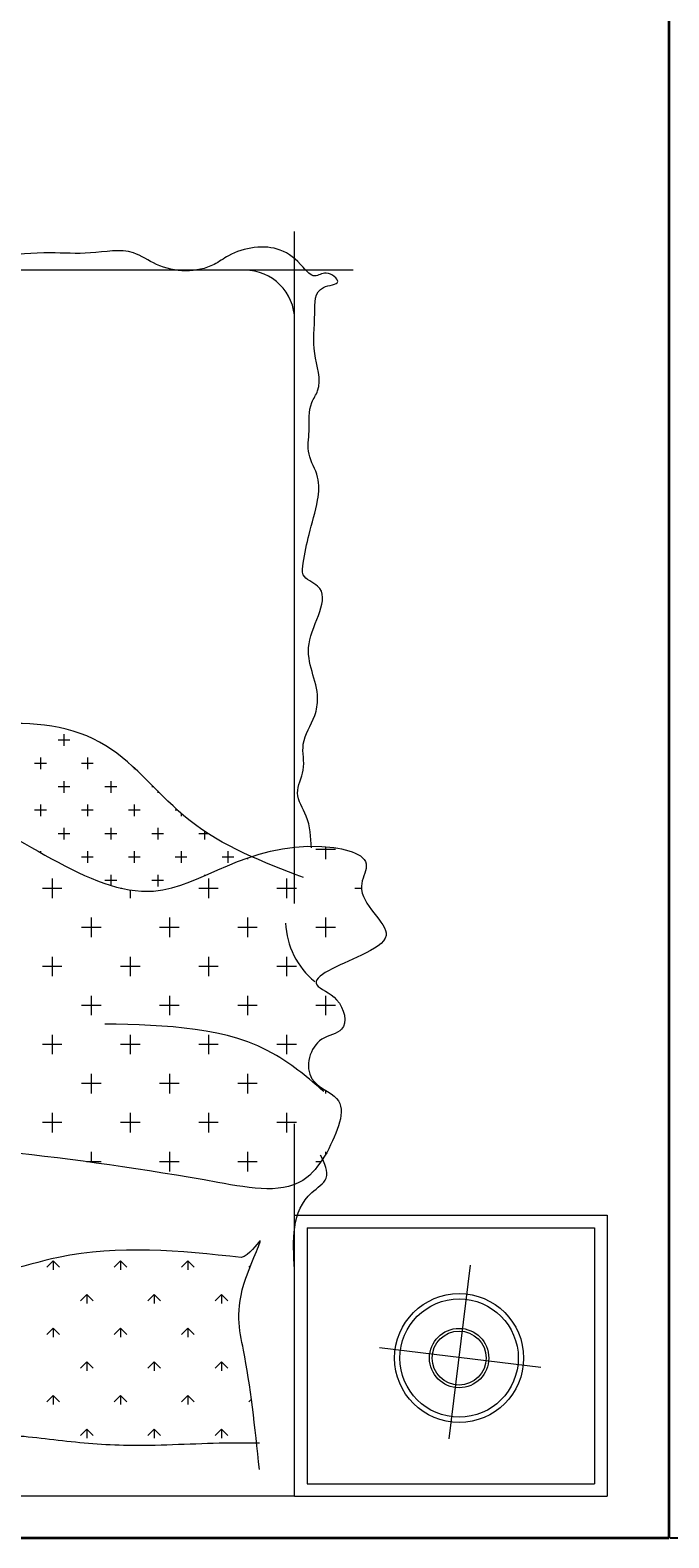
# Model space of a CAD drawing. Units: inches. Extents: x 3731 to 4318, y 1310 to 2388.
# Tile 46 of 57: x 4192 to 4234, y 1943 to 2043. Entities that reach past the tile are written whole.
import ezdxf

# ---------------------------------------------------------------- set-up
doc = ezdxf.new("R2010")
doc.units = ezdxf.units.IN
for name, color, linetype, lineweight in [('A-ANNO-DIMS', 2, 'Continuous', 18), ('A-FURN', 8, 'Continuous', 13), ('A-WALL', 7, 'Continuous', 35)]:
    doc.layers.add(name, color=color, linetype=linetype, lineweight=lineweight)
doc.styles.get("Standard").update_dxf_attribs({"font": 'arial.ttf'})
doc.dimstyles.get("Standard").update_dxf_attribs({"dimtxt": 0.18, "dimasz": 0.18, "dimexe": 0.18, "dimexo": 0.0625, "dimgap": 0.09, "dimtad": 0, "dimtih": 1, "dimtoh": 1, "dimdec": 4, "dimzin": 0, "dimdsep": 46, "dimtxsty": 'Standard', "dimcen": 0.09, "dimadec": 0, "dimazin": 0, "dimtfac": 1, "dimtdec": 4, "dimtofl": 0, "dimtmove": 0, "dimatfit": 3, "dimfxl": 1, "dimtolj": 1, "dimtzin": 0, "dimarcsym": 0})

# ---------------------------------------------------------------- blocks, each defined once
blk = doc.blocks.new('A$C200C7901')
for p, q in [((0, 1.8834), (0, 2.3334)), ((0.5, 2.3334), (0, 2.3334)), ((0.5, 2.3334), (0.5, 1.7369)), ((0.5, 2.3334), (0.5, 1.7369)), ((0.5, 2.3334), (2, 2.3334)), ((0.5701, 1.9635), (0.5733, 1.9666)), ((0.5701, 1.9635), (0.5733, 1.9666)), ((0.5, 1.8834), (0, 1.8834)), ((0.4504, 1.782), (0.4504, 1.7863)), ((0.4504, 1.782), (0.4504, 1.7863)), ((0.458, 1.7977), (0.466, 1.7977)), ((0.458, 1.7977), (0.466, 1.7977)), ((0.4504, 1.6834), (0.4504, 1.6883)), ((0.4504, 1.6834), (0.4504, 1.6883)), ((0.4656, 1.6727), (0.466, 1.6727)), ((0.4656, 1.6727), (0.466, 1.6727)), ((0.5597, 1.6727), (0.591, 1.6727)), ((0.5597, 1.6727), (0.591, 1.6727)), ((0.4347, 1.5477), (0.466, 1.5477)), ((0.4504, 1.532), (0.4504, 1.5633)), ((0.6847, 1.5477), (0.716, 1.5477)), ((0.4347, 1.4227), (0.466, 1.4227)), ((0.5, 1.3845), (0.5, 0.3086)), ((0.3931, 1.3602), (0.4035, 1.3602)), ((0.3931, 1.3602), (0.4035, 1.3602)), ((0.4972, 1.3602), (0.5285, 1.3602)), ((0.4972, 1.3602), (0.5285, 1.3602)), ((0.4504, 1.2936), (0.4504, 1.3133)), ((0.4504, 1.2936), (0.4504, 1.3133)), ((0.4347, 1.2977), (0.466, 1.2977)), ((0.4347, 1.2977), (0.466, 1.2977)), ((0.4061, 0.3703), (2.0386, 0.3703))]:
    blk.add_line(p, q)
at = {"linetype": 'ByBlock'}
for p, q in [((0.02, 1.9034), (0.02, 2.3134)), ((0.48, 2.3134), (0.02, 2.3134)), ((0.48, 1.9034), (0.48, 2.3134)), ((0.2524, 2.2412), (0.2186, 1.9635)), ((0.6171, 2.2259), (0.607, 2.236)), ((0.6171, 2.2259), (0.607, 2.236)), ((0.6171, 2.2259), (0.6171, 2.2402)), ((0.6171, 2.2259), (0.6171, 2.2402)), ((0.6171, 2.2259), (0.6272, 2.236)), ((0.6171, 2.2259), (0.6272, 2.236)), ((0.7249, 2.2259), (0.7148, 2.236)), ((0.7249, 2.2259), (0.7148, 2.236)), ((0.7249, 2.2259), (0.7249, 2.2402)), ((0.7249, 2.2259), (0.7249, 2.2402)), ((0.7249, 2.2259), (0.735, 2.236)), ((0.7249, 2.2259), (0.735, 2.236)), ((0.8326, 2.2259), (0.8225, 2.236)), ((0.8326, 2.2259), (0.8225, 2.236)), ((0.8326, 2.2259), (0.8326, 2.2402)), ((0.8326, 2.2259), (0.8326, 2.2402)), ((0.8326, 2.2259), (0.8427, 2.236)), ((0.8326, 2.2259), (0.8427, 2.236)), ((0.5692, 2.178), (0.5733, 2.1822)), ((0.5692, 2.178), (0.5733, 2.1822)), ((0.671, 2.1721), (0.6609, 2.1822)), ((0.671, 2.1721), (0.6609, 2.1822)), ((0.671, 2.172), (0.671, 2.1863)), ((0.671, 2.172), (0.671, 2.1863)), ((0.671, 2.1721), (0.6811, 2.1822)), ((0.671, 2.1721), (0.6811, 2.1822)), ((0.7787, 2.1721), (0.7686, 2.1822)), ((0.7787, 2.1721), (0.7686, 2.1822)), ((0.7787, 2.172), (0.7787, 2.1863)), ((0.7787, 2.172), (0.7787, 2.1863)), ((0.7787, 2.1721), (0.7889, 2.1822)), ((0.7787, 2.1721), (0.7889, 2.1822)), ((0.8865, 2.1721), (0.8764, 2.1822)), ((0.8865, 2.1721), (0.8764, 2.1822)), ((0.8865, 2.172), (0.8865, 2.1863)), ((0.8865, 2.172), (0.8865, 2.1863)), ((0.8865, 2.1721), (0.8966, 2.1822)), ((0.8865, 2.1721), (0.8966, 2.1822)), ((0.3641, 2.0951), (0.1061, 2.1268)), ((0.6171, 2.1182), (0.607, 2.1283)), ((0.6171, 2.1182), (0.607, 2.1283)), ((0.6171, 2.1182), (0.6171, 2.1325)), ((0.6171, 2.1182), (0.6171, 2.1325)), ((0.6171, 2.1182), (0.6272, 2.1283)), ((0.6171, 2.1182), (0.6272, 2.1283)), ((0.7249, 2.1182), (0.7148, 2.1283)), ((0.7249, 2.1182), (0.7148, 2.1283)), ((0.7249, 2.1182), (0.7249, 2.1325)), ((0.7249, 2.1182), (0.7249, 2.1325)), ((0.7249, 2.1182), (0.735, 2.1283)), ((0.7249, 2.1182), (0.735, 2.1283)), ((0.8326, 2.1182), (0.8225, 2.1283)), ((0.8326, 2.1182), (0.8225, 2.1283)), ((0.8326, 2.1182), (0.8326, 2.1325)), ((0.8326, 2.1182), (0.8326, 2.1325)), ((0.8326, 2.1182), (0.8427, 2.1283)), ((0.8326, 2.1182), (0.8427, 2.1283)), ((0.671, 2.0643), (0.671, 2.0786)), ((0.671, 2.0643), (0.671, 2.0786)), ((0.7787, 2.0643), (0.7787, 2.0786)), ((0.7787, 2.0643), (0.7787, 2.0786)), ((0.8865, 2.0643), (0.8865, 2.0786)), ((0.8865, 2.0643), (0.8865, 2.0786)), ((0.671, 2.0643), (0.6609, 2.0744)), ((0.671, 2.0643), (0.6609, 2.0744)), ((0.671, 2.0643), (0.6811, 2.0744)), ((0.671, 2.0643), (0.6811, 2.0744)), ((0.7787, 2.0643), (0.7686, 2.0744)), ((0.7787, 2.0643), (0.7686, 2.0744)), ((0.7787, 2.0643), (0.7889, 2.0744)), ((0.7787, 2.0643), (0.7889, 2.0744)), ((0.8865, 2.0643), (0.8764, 2.0744)), ((0.8865, 2.0643), (0.8764, 2.0744)), ((0.8865, 2.0643), (0.8966, 2.0744)), ((0.8865, 2.0643), (0.8966, 2.0744)), ((0.6171, 2.0104), (0.607, 2.0205)), ((0.6171, 2.0104), (0.607, 2.0205)), ((0.6171, 2.0104), (0.6171, 2.0247)), ((0.6171, 2.0104), (0.6171, 2.0247)), ((0.6171, 2.0104), (0.6272, 2.0205)), ((0.6171, 2.0104), (0.6272, 2.0205)), ((0.7249, 2.0104), (0.7148, 2.0205)), ((0.7249, 2.0104), (0.7148, 2.0205)), ((0.7249, 2.0104), (0.7249, 2.0247)), ((0.7249, 2.0104), (0.7249, 2.0247)), ((0.7249, 2.0104), (0.735, 2.0205)), ((0.7249, 2.0104), (0.735, 2.0205)), ((0.8326, 2.0104), (0.8225, 2.0205)), ((0.8326, 2.0104), (0.8225, 2.0205)), ((0.8326, 2.0104), (0.8326, 2.0247)), ((0.8326, 2.0104), (0.8326, 2.0247)), ((0.8326, 2.0104), (0.8427, 2.0205)), ((0.8326, 2.0104), (0.8427, 2.0205)), ((0.671, 1.9565), (0.6609, 1.9666)), ((0.671, 1.9565), (0.6609, 1.9666)), ((0.671, 1.9565), (0.671, 1.9708)), ((0.671, 1.9565), (0.671, 1.9708)), ((0.671, 1.9565), (0.6811, 1.9666)), ((0.671, 1.9565), (0.6811, 1.9666)), ((0.7787, 1.9565), (0.7686, 1.9666)), ((0.7787, 1.9565), (0.7686, 1.9666)), ((0.7787, 1.9565), (0.7787, 1.9708)), ((0.7787, 1.9565), (0.7787, 1.9708)), ((0.7787, 1.9565), (0.7889, 1.9666)), ((0.7787, 1.9565), (0.7889, 1.9666)), ((0.8865, 1.9565), (0.8764, 1.9666)), ((0.8865, 1.9565), (0.8764, 1.9666)), ((0.8865, 1.9565), (0.8865, 1.9708)), ((0.8865, 1.9565), (0.8865, 1.9708)), ((0.8865, 1.9565), (0.8966, 1.9666)), ((0.8865, 1.9565), (0.8966, 1.9666)), ((0.48, 1.9034), (0.02, 1.9034)), ((0.5754, 1.782), (0.5754, 1.8133)), ((0.5754, 1.782), (0.5754, 1.8133)), ((0.7004, 1.782), (0.7004, 1.8133)), ((0.7004, 1.782), (0.7004, 1.8133)), ((0.5597, 1.7977), (0.591, 1.7977)), ((0.5597, 1.7977), (0.591, 1.7977)), ((0.6847, 1.7977), (0.716, 1.7977)), ((0.6847, 1.7977), (0.716, 1.7977)), ((0.8097, 1.7977), (0.8331, 1.7977)), ((0.8097, 1.7977), (0.8331, 1.7977)), ((0.8254, 1.782), (0.8254, 1.7987)), ((0.8254, 1.782), (0.8254, 1.7987)), ((0.5129, 1.7195), (0.5129, 1.7508)), ((0.5129, 1.7195), (0.5129, 1.7508)), ((0.6379, 1.7195), (0.6379, 1.7508)), ((0.6379, 1.7195), (0.6379, 1.7508)), ((0.7629, 1.7195), (0.7629, 1.7508)), ((0.7629, 1.7195), (0.7629, 1.7508)), ((0.8879, 1.7195), (0.8879, 1.7508)), ((0.8879, 1.7195), (0.8879, 1.7508)), ((0.4972, 1.7352), (0.5285, 1.7352)), ((0.4972, 1.7352), (0.5285, 1.7352)), ((0.6222, 1.7352), (0.6535, 1.7352)), ((0.6222, 1.7352), (0.6535, 1.7352)), ((0.7472, 1.7352), (0.7785, 1.7352)), ((0.7472, 1.7352), (0.7785, 1.7352)), ((0.8722, 1.7352), (0.9035, 1.7352)), ((0.8722, 1.7352), (0.9035, 1.7352)), ((0.5754, 1.657), (0.5754, 1.6883)), ((0.5754, 1.657), (0.5754, 1.6883)), ((0.6847, 1.6727), (0.716, 1.6727)), ((0.6847, 1.6727), (0.716, 1.6727)), ((0.7004, 1.657), (0.7004, 1.6883)), ((0.7004, 1.657), (0.7004, 1.6883)), ((0.8097, 1.6727), (0.841, 1.6727)), ((0.8097, 1.6727), (0.841, 1.6727)), ((0.8254, 1.657), (0.8254, 1.6883)), ((0.8254, 1.657), (0.8254, 1.6883)), ((0.5129, 1.5945), (0.5129, 1.6258)), ((0.5129, 1.5945), (0.5129, 1.6258)), ((0.6379, 1.5945), (0.6379, 1.6258)), ((0.6379, 1.5945), (0.6379, 1.6258)), ((0.7629, 1.5945), (0.7629, 1.6258)), ((0.7629, 1.5945), (0.7629, 1.6258)), ((0.8879, 1.5945), (0.8879, 1.6258)), ((0.8879, 1.5945), (0.8879, 1.6258)), ((0.4972, 1.6102), (0.5285, 1.6102)), ((0.4972, 1.6102), (0.5285, 1.6102)), ((0.6222, 1.6102), (0.6535, 1.6102)), ((0.6222, 1.6102), (0.6535, 1.6102)), ((0.7472, 1.6102), (0.7785, 1.6102)), ((0.7472, 1.6102), (0.7785, 1.6102)), ((0.8722, 1.6102), (0.9035, 1.6102)), ((0.8722, 1.6102), (0.9035, 1.6102)), ((0.4347, 1.5477), (0.466, 1.5477)), ((0.4504, 1.532), (0.4504, 1.5633)), ((0.5597, 1.5477), (0.591, 1.5477)), ((0.5597, 1.5477), (0.591, 1.5477)), ((0.5754, 1.532), (0.5754, 1.5633)), ((0.5754, 1.532), (0.5754, 1.5633)), ((0.6847, 1.5477), (0.716, 1.5477)), ((0.7004, 1.532), (0.7004, 1.5633)), ((0.7004, 1.532), (0.7004, 1.5633)), ((0.8097, 1.5477), (0.841, 1.5477)), ((0.8097, 1.5477), (0.841, 1.5477)), ((0.8254, 1.532), (0.8254, 1.5633)), ((0.8254, 1.532), (0.8254, 1.5633)), ((0.5129, 1.4695), (0.5129, 1.5008)), ((0.5129, 1.4695), (0.5129, 1.5008)), ((0.6379, 1.4695), (0.6379, 1.5008)), ((0.6379, 1.4695), (0.6379, 1.5008)), ((0.7629, 1.4695), (0.7629, 1.5008)), ((0.7629, 1.4695), (0.7629, 1.5008)), ((0.8879, 1.4695), (0.8879, 1.5008)), ((0.8879, 1.4695), (0.8879, 1.5008)), ((0.4972, 1.4852), (0.5285, 1.4852)), ((0.4972, 1.4852), (0.5285, 1.4852)), ((0.6222, 1.4852), (0.6535, 1.4852)), ((0.6222, 1.4852), (0.6535, 1.4852)), ((0.7472, 1.4852), (0.7785, 1.4852)), ((0.7472, 1.4852), (0.7785, 1.4852)), ((0.8722, 1.4852), (0.9035, 1.4852)), ((0.8722, 1.4852), (0.9035, 1.4852)), ((0.4504, 1.407), (0.4504, 1.4383)), ((0.4504, 1.407), (0.4504, 1.4383)), ((0.5754, 1.407), (0.5754, 1.4383)), ((0.5754, 1.407), (0.5754, 1.4383)), ((0.7004, 1.407), (0.7004, 1.4383)), ((0.7004, 1.407), (0.7004, 1.4383)), ((0.8254, 1.407), (0.8254, 1.4383)), ((0.8254, 1.407), (0.8254, 1.4383)), ((0.4347, 1.4227), (0.466, 1.4227)), ((0.5597, 1.4227), (0.591, 1.4227)), ((0.5597, 1.4227), (0.591, 1.4227)), ((0.6847, 1.4227), (0.716, 1.4227)), ((0.6847, 1.4227), (0.716, 1.4227)), ((0.8097, 1.4227), (0.841, 1.4227)), ((0.8097, 1.4227), (0.841, 1.4227)), ((0.5129, 1.3445), (0.5129, 1.3758)), ((0.5129, 1.3445), (0.5129, 1.3758)), ((0.6222, 1.3602), (0.6535, 1.3602)), ((0.6222, 1.3602), (0.6535, 1.3602)), ((0.6379, 1.3445), (0.6379, 1.3758)), ((0.6379, 1.3445), (0.6379, 1.3758)), ((0.7191, 1.3383), (0.7191, 1.357)), ((0.7191, 1.3383), (0.7191, 1.357)), ((0.7629, 1.3627), (0.7629, 1.3758)), ((0.7629, 1.3627), (0.7629, 1.3758)), ((0.7762, 1.3602), (0.7785, 1.3602)), ((0.7762, 1.3602), (0.7785, 1.3602)), ((0.7941, 1.3383), (0.7941, 1.3554)), ((0.7941, 1.3383), (0.7941, 1.3554)), ((0.8722, 1.3602), (0.9035, 1.3602)), ((0.8722, 1.3602), (0.9035, 1.3602)), ((0.8879, 1.3445), (0.8879, 1.3758)), ((0.8879, 1.3445), (0.8879, 1.3758)), ((0.6441, 1.3383), (0.6441, 1.3399)), ((0.6441, 1.3383), (0.6441, 1.3399)), ((0.7097, 1.3477), (0.7285, 1.3477)), ((0.7097, 1.3477), (0.7285, 1.3477)), ((0.7847, 1.3477), (0.8035, 1.3477)), ((0.7847, 1.3477), (0.8035, 1.3477)), ((0.5754, 1.3115), (0.5754, 1.3133)), ((0.5754, 1.3115), (0.5754, 1.3133)), ((0.5972, 1.3102), (0.616, 1.3102)), ((0.5972, 1.3102), (0.616, 1.3102)), ((0.6066, 1.3008), (0.6066, 1.3195)), ((0.6066, 1.3008), (0.6066, 1.3195)), ((0.6722, 1.3102), (0.691, 1.3102)), ((0.6722, 1.3102), (0.691, 1.3102)), ((0.6816, 1.3008), (0.6816, 1.3195)), ((0.6816, 1.3008), (0.6816, 1.3195)), ((0.7472, 1.3102), (0.766, 1.3102)), ((0.7472, 1.3102), (0.766, 1.3102)), ((0.7566, 1.3008), (0.7566, 1.3195)), ((0.7566, 1.3008), (0.7566, 1.3195)), ((0.8222, 1.3102), (0.841, 1.3102)), ((0.8222, 1.3102), (0.841, 1.3102)), ((0.8316, 1.3008), (0.8316, 1.3195)), ((0.8316, 1.3008), (0.8316, 1.3195)), ((0.6441, 1.2686), (0.6441, 1.282)), ((0.6441, 1.2686), (0.6441, 1.282)), ((0.7191, 1.2633), (0.7191, 1.282)), ((0.7191, 1.2633), (0.7191, 1.282)), ((0.7941, 1.2633), (0.7941, 1.282)), ((0.7941, 1.2633), (0.7941, 1.282)), ((0.8691, 1.2633), (0.8691, 1.282)), ((0.8691, 1.2633), (0.8691, 1.282)), ((0.9066, 1.3008), (0.9066, 1.3028)), ((0.9066, 1.3008), (0.9066, 1.3028)), ((0.6379, 1.2727), (0.6535, 1.2727)), ((0.6379, 1.2727), (0.6535, 1.2727)), ((0.7097, 1.2727), (0.7285, 1.2727)), ((0.7097, 1.2727), (0.7285, 1.2727)), ((0.7847, 1.2727), (0.8035, 1.2727)), ((0.7847, 1.2727), (0.8035, 1.2727)), ((0.8597, 1.2727), (0.8785, 1.2727)), ((0.8597, 1.2727), (0.8785, 1.2727)), ((0.6816, 1.2398), (0.6816, 1.2445)), ((0.6816, 1.2398), (0.6816, 1.2445)), ((0.6868, 1.2352), (0.691, 1.2352)), ((0.6868, 1.2352), (0.691, 1.2352)), ((0.7472, 1.2352), (0.766, 1.2352)), ((0.7472, 1.2352), (0.766, 1.2352)), ((0.7566, 1.2258), (0.7566, 1.2445)), ((0.7566, 1.2258), (0.7566, 1.2445)), ((0.8222, 1.2352), (0.841, 1.2352)), ((0.8222, 1.2352), (0.841, 1.2352)), ((0.8316, 1.2258), (0.8316, 1.2445)), ((0.8316, 1.2258), (0.8316, 1.2445)), ((0.8972, 1.2352), (0.916, 1.2352)), ((0.8972, 1.2352), (0.916, 1.2352)), ((0.9066, 1.2258), (0.9066, 1.2445)), ((0.9066, 1.2258), (0.9066, 1.2445)), ((0.7191, 1.2041), (0.7191, 1.207)), ((0.7191, 1.2041), (0.7191, 1.207)), ((0.7941, 1.1883), (0.7941, 1.207)), ((0.7941, 1.1883), (0.7941, 1.207)), ((0.8691, 1.1883), (0.8691, 1.207)), ((0.8691, 1.1883), (0.8691, 1.207)), ((0.7255, 1.1977), (0.7285, 1.1977)), ((0.7255, 1.1977), (0.7285, 1.1977)), ((0.7847, 1.1977), (0.8035, 1.1977)), ((0.7847, 1.1977), (0.8035, 1.1977)), ((0.8597, 1.1977), (0.8785, 1.1977)), ((0.8597, 1.1977), (0.8785, 1.1977)), ((0.7566, 1.1674), (0.7566, 1.1695)), ((0.7566, 1.1674), (0.7566, 1.1695)), ((0.7646, 1.1602), (0.766, 1.1602)), ((0.7646, 1.1602), (0.766, 1.1602)), ((0.8222, 1.1602), (0.841, 1.1602)), ((0.8222, 1.1602), (0.841, 1.1602)), ((0.8316, 1.1508), (0.8316, 1.1695)), ((0.8316, 1.1508), (0.8316, 1.1695)), ((0.8972, 1.1602), (0.916, 1.1602)), ((0.8972, 1.1602), (0.916, 1.1602)), ((0.9066, 1.1508), (0.9066, 1.1695)), ((0.9066, 1.1508), (0.9066, 1.1695)), ((0.8597, 1.1227), (0.8785, 1.1227)), ((0.8597, 1.1227), (0.8785, 1.1227)), ((0.8691, 1.1133), (0.8691, 1.132)), ((0.8691, 1.1133), (0.8691, 1.132))]:
    blk.add_line(p, q, dxfattribs=at)
for radius in [0.1032, 0.0947, 0.0475, 0.0432]:
    blk.add_circle((0.2367, 2.1121), radius, dxfattribs=at)
blk.add_arc((0.3888, 1.4113), 0.1256, 1.9962, 51.1646, dxfattribs=at)
for centre, radius, start, end in [((0.3888, 1.4113), 0.1256, 1.9962, 51.1646), ((0.58, 0.4503), 0.08, 180, 270)]:
    blk.add_arc(centre, radius, start, end)
for points, knots in [([(0.5562, 2.2908), (0.5634, 2.223), (0.5751, 2.1147), (0.6005, 2.0213), (0.5392, 1.8966), (0.5726, 1.9486), (0.5854, 1.951)], [0, 0, 0, 0, 193.119101, 308.278592, 371.468985, 410.593498, 410.593498, 410.593498, 410.593498]), ([(0.5854, 1.951), (0.6835, 1.9407), (0.8425, 1.9242), (1.0374, 2.0054), (1.1564, 1.9255), (1.2274, 1.9841), (1.2052, 2.0751), (1.1815, 2.152), (1.2176, 2.2368), (1.0992, 2.2731), (1.0008, 2.2255), (0.8698, 2.246), (0.7481, 2.2548), (0.6426, 2.2473), (0.5746, 2.2478), (0.5562, 2.2479)], [0, 0, 0, 0, 292.165466, 473.33038, 601.631673, 630.723769, 727.138505, 836.819956, 887.958136, 954.42438, 1118.989809, 1227.016542, 1338.750986, 1487.447361, 1542.751028, 1542.751028, 1542.751028, 1542.751028]), ([(0.4485, 1.7835), (0.4321, 1.7496), (0.4062, 1.6964), (0.49, 1.6713), (0.4719, 1.5969), (0.4123, 1.592), (0.4233, 1.5337), (0.4954, 1.5086), (0.4012, 1.4738), (0.3253, 1.4306), (0.4113, 1.3764), (0.3688, 1.3065), (0.5579, 1.2663), (0.741, 1.4533), (1.1127, 1.1109), (1.4811, 1.2478), (1.7885, 1.3492), (2.0357, 1.1637), (2.0748, 1.2974), (2.0876, 1.349), (2.0192, 1.3805), (2.0564, 1.4298), (2.0588, 1.4846), (1.9759, 1.5349), (2.1004, 1.5845), (2.0397, 1.6519), (1.971, 1.7053), (2.1104, 1.8981), (1.5946, 1.7967), (1.2448, 1.7472), (0.8129, 1.7935), (0.4953, 1.8548), (0.4582, 1.7983), (0.4485, 1.7835)], [0, 0, 0, 0, 88.420092, 139.08588, 204.302936, 239.695496, 287.801042, 327.365471, 412.960499, 463.626286, 552.059846, 584.668336, 662.614915, 940.993281, 1309.926334, 1844.022653, 1996.276242, 2316.43048, 2341.441004, 2404.707416, 2449.463774, 2514.680778, 2538.40571, 2613.031547, 2697.13096, 2760.903931, 2822.692699, 2945.47, 3215.060018, 3725.584917, 4361.974444, 4504.671998, 4555.32777, 4555.32777, 4555.32777, 4555.32777]), ([(0.4856, 1.3429), (0.5504, 1.3182), (0.6715, 1.2721), (0.8374, 1.0498), (1.1164, 1.1183), (1.3878, 1.1816), (1.5888, 1.1102), (1.8403, 1.1127), (1.9415, 1.2178), (2.0032, 1.2819)], [0, 0, 0, 0, 205.411753, 383.654933, 772.067458, 921.644661, 1226.793228, 1388.983508, 1642.292305, 1642.292305, 1642.292305, 1642.292305])]:
    blk.add_open_spline(points, degree=3, knots=knots)
for points, knots in [([(0.5, 1.9703), (0.5029, 1.9235), (0.5066, 1.8648), (0.4398, 1.8252), (0.452, 1.8005), (0.4585, 1.7872)], [0, 0, 0, 0, 126.315232, 158.854004, 196.789047, 196.789047, 196.789047, 196.789047]), ([(0.5, 1.9703), (0.5029, 1.9235), (0.5066, 1.8648), (0.4398, 1.8252), (0.452, 1.8005), (0.4585, 1.7872)], [0, 0, 0, 0, 126.315232, 158.854004, 196.789047, 196.789047, 196.789047, 196.789047]), ([(0.4532, 1.6853), (0.4776, 1.6644), (0.574, 1.582), (0.7055, 1.5794), (0.8037, 1.5774)], [0, 0, 0, 0, 94.920667, 374.457292, 374.457292, 374.457292, 374.457292]), ([(0.4532, 1.6853), (0.4776, 1.6644), (0.574, 1.582), (0.7055, 1.5794), (0.8037, 1.5774)], [0, 0, 0, 0, 94.920667, 374.457292, 374.457292, 374.457292, 374.457292]), ([(0.473, 1.2954), (0.4739, 1.2781), (0.4755, 1.2477), (0.5032, 1.2084), (0.4801, 1.1701), (0.4928, 1.1255), (0.4674, 1.0912), (0.4579, 1.0351), (0.501, 0.9724), (0.4311, 0.8832), (0.4902, 0.8637), (0.4843, 0.8288), (0.4774, 0.7906), (0.4625, 0.7457), (0.459, 0.6999), (0.4816, 0.6664), (0.4748, 0.625), (0.4791, 0.5889), (0.4533, 0.5528), (0.4738, 0.5004), (0.4658, 0.4502), (0.4696, 0.3946), (0.4189, 0.3935), (0.4493, 0.3684), (0.4694, 0.3857), (0.4922, 0.3576), (0.5297, 0.3262), (0.5917, 0.3353), (0.6454, 0.3754), (0.7083, 0.3741), (0.7643, 0.3328), (0.826, 0.346), (0.925, 0.3388), (1.0353, 0.3593), (1.1561, 0.3744), (1.2477, 0.3154), (1.3302, 0.3474), (1.4086, 0.3512), (1.5217, 0.3878), (1.6362, 0.3176), (1.7682, 0.3285), (1.8402, 0.3019), (1.9071, 0.3529), (1.9647, 0.3412), (2.0795, 0.2948), (2.0472, 0.3498), (2.0343, 0.3772), (2.0435, 0.43), (2.0109, 0.5782), (2.0746, 0.4643), (2.0805, 0.584), (2.0084, 0.5979), (2.0343, 0.6846), (2.0344, 0.746), (2.0293, 0.8096), (2.0489, 0.8545), (2.0652, 0.9218), (1.9842, 0.9297), (2.0007, 1.0162), (2.0367, 1.0585), (2.0367, 1.1102), (2.0457, 1.1647), (2.0226, 1.2084), (2.0234, 1.2306), (2.0236, 1.2352)], [0, 0, 0, 0, 51.660678, 90.967412, 128.902454, 170.303599, 219.852997, 247.834962, 336.321557, 429.35469, 458.821847, 477.222321, 524.135809, 581.038434, 617.839381, 657.146115, 693.947125, 740.178081, 760.753248, 820.731705, 885.133458, 928.777044, 953.563729, 976.574207, 995.553042, 1018.563482, 1064.584401, 1147.951297, 1174.787598, 1266.851571, 1308.018447, 1377.066427, 1441.511314, 1608.245014, 1714.11869, 1792.771707, 1913.247991, 1954.931389, 2029.864445, 2259.189419, 2305.221512, 2429.507982, 2456.344283, 2543.92595, 2627.925037, 2662.96218, 2687.736879, 2719.937755, 2839.540991, 2875.47895, 2953.681041, 2993.270313, 3066.872333, 3154.395764, 3200.397042, 3248.426375, 3312.828127, 3347.881398, 3444.484026, 3481.577522, 3518.665244, 3592.267265, 3644.719162, 3658.519501, 3658.519501, 3658.519501, 3658.519501])]:
    blk.add_open_spline(points, degree=3, knots=knots, dxfattribs=at)
blk = doc.blocks.new('*D38')
at = {"layer": 'A-ANNO-DIMS', "color": 0, "lineweight": -2, "transparency": 16777216}
for p, q in [((4103.271, 2262.382), (4318.341, 2262.382)), ((4318.161, 2262.202), (4318.161, 2103.064)), ((4318.161, 1943.562), (4318.161, 2102.7)), ((4234.271, 1943.382), (4318.341, 1943.382))]:
    blk.add_line(p, q, dxfattribs=at)
at = {"layer": 'A-ANNO-DIMS', "color": 0, "transparency": 16777216}
for points in [[(4318.131, 2262.202), (4318.191, 2262.202), (4318.161, 2262.382)], [(4318.131, 1943.562), (4318.191, 1943.562), (4318.161, 1943.382)]]:
    blk.add_solid(points, dxfattribs=at)
at = {"layer": 'Defpoints', "color": 0, "transparency": 16777216}
for p in [(4103.209, 2262.382), (4318.161, 2262.382), (4234.209, 1943.382)]:
    blk.add_point(p, dxfattribs=at)
at = {"layer": 'A-ANNO-DIMS', "color": 0, "transparency": 16777216, "insert": (4318.161, 2102.882), "char_height": 0.18, "attachment_point": 5}
blk.add_mtext('\\A1;319', dxfattribs=at)

msp = doc.modelspace()

# ---------------------------------------------------------------- linework, layer by layer
at = {"layer": 'A-WALL'}
for p in [(4234.209, 2069.382), (4108.209, 1943.382)]:
    msp.add_line(p, (4234.209, 1943.382), dxfattribs=at)

# ---------------------------------------------------------------- block references
at = {"layer": 'A-FURN', "xscale": 41.1071563136412, "yscale": 41.1071563136412, "zscale": 41.1071563136412, "rotation": 180}
msp.add_blockref('A$C200C7901', (4230.145, 2042.037), dxfattribs=at)

# ---------------------------------------------------------------- dimensions: what is measured, and where the dimension line sits
at = {"layer": 'A-ANNO-DIMS'}
dim = msp.add_linear_dim(base=(4318.161, 2262.382), p1=(4234.209, 1943.382), p2=(4103.209, 2262.382), angle=90, dimstyle='Standard', override={"dimdec": 0, "dimlfac": 1, "dimrnd": 0, "dimzin": 0, "dimdsep": 46, "dimlunit": 2}, dxfattribs=at)
dim.commit()
dim.dimension.update_dxf_attribs({"geometry": '*D38', "text_midpoint": (4318.161, 2102.882)})

doc.saveas('drawing.dxf')
